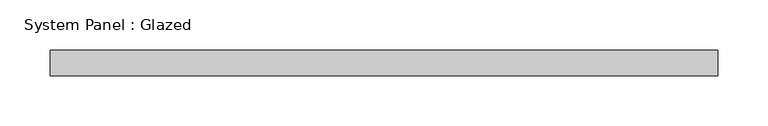
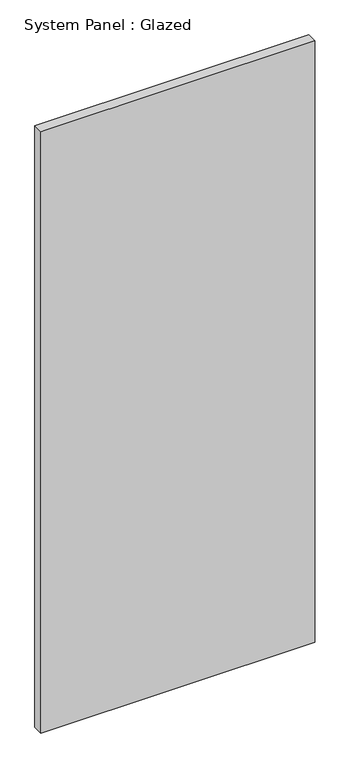
"""IFC4 building model written with IfcOpenShell, lengths in millimetres: plate geometry, System Panel : Glazed."""

from ifc_helpers import new_model, si_unit, origin, origin_with_axes, place, context, project, spatial, polyline, outline, extrude, source, transform, mapped, element, save


def system_panel_glazed_25c2e5f5(model_context):
    return source(origin(), model_context, "Body", "SweptSolid", [
        extrude(outline(polyline([(333.375, 19.05), (-333.375, 19.05), (-333.375, 44.45), (333.375, 44.45), (333.375, 19.05)])), origin_with_axes(), (0.0, 0.0, 1.0), 1548.41517),
    ])


if __name__ == "__main__":
    model = new_model("IFC4")
    model_context = context("Model", 3, world=origin())
    ifc_project = project(units=[si_unit("LENGTHUNIT", "METRE", prefix="MILLI")], contexts=[model_context])
    site = spatial("IfcSite", under=ifc_project)
    building = spatial("IfcBuilding", under=site)
    placement = place(None, origin())
    system_panel_glazed_shape = system_panel_glazed_25c2e5f5(model_context)
    element("IfcPlate", 1, ObjectType="System Panel : Glazed", at=placement, inside=building, context=model_context, shape_type="MappedRepresentation", body=[
        mapped(system_panel_glazed_shape, transform((0.0, 0.0, 0.0), x_axis=(1.0, 0.0, 0.0), y_axis=(0.0, 1.0, 0.0), z_axis=(0.0, 0.0, 1.0))),
    ])
    save(model, "model.ifc")

# Revit data of these elements
# Type "System Panel : Glazed"
#   Construction Type Id = "GSP4R"
#   Analytic Construction = "1/8 in Pilkington single glazing"
#   Visual Light Transmittance = 0.9
#   Solar Heat Gain Coefficient = 0.86
#   Heat Transfer Coefficient (U) = 1.18115 BTU/(h·ft²·°F)
#   Define Thermal Properties by = 1
# Element 1 (IfcPlate, "System Panel : Glazed")
#   Materials on its faces: "Glass"
# Materials
#   "Glass": class "Glass", colour RGB 0 128 192, transparency 0.75, Description = "Soda Lime Glass", Cost = 0
